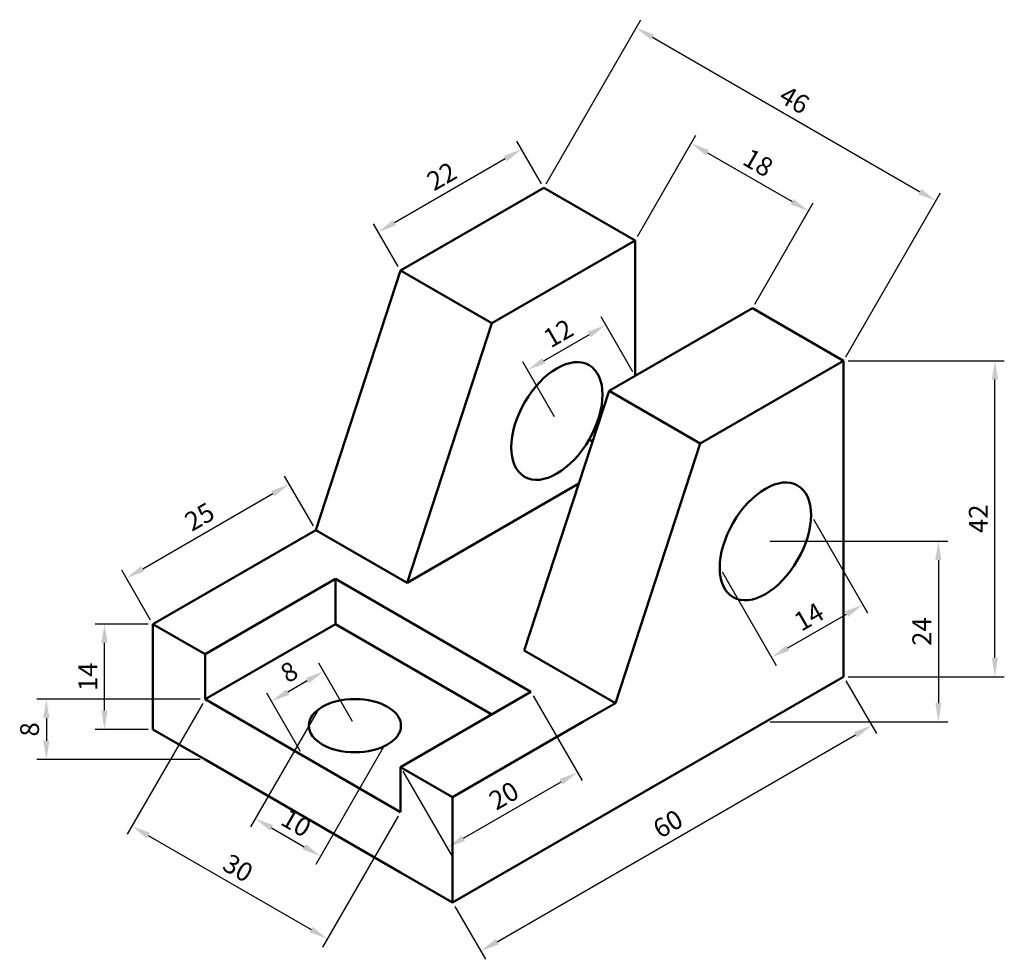
# Model space of a CAD drawing. Units: millimetres. Extents: x 1547 to 1678, y 118 to 243.
import ezdxf

# ---------------------------------------------------------------- set-up
doc = ezdxf.new("R2010")
doc.units = ezdxf.units.MM
doc.layers.add('M-DIMS', color=2, linetype='Continuous', lineweight=25)
doc.layers.add('M-OUTL', color=7, linetype='Continuous', lineweight=50)
doc.styles.get("Standard").update_dxf_attribs({"font": 'arial.ttf'})
doc.dimstyles.new('ISO-25', dxfattribs={"dimtxt": 2.5, "dimasz": 2.5, "dimexe": 1.25, "dimexo": 0.625, "dimtad": 1, "dimtxsty": 'Standard', "dimcen": 2.5, "dimadec": 0, "dimazin": 0, "dimtfac": 1, "dimtmove": 0, "dimatfit": 3, "dimfxl": 1, "dimarcsym": 0})

# ---------------------------------------------------------------- blocks, each defined once
blk = doc.blocks.new('*D1')
at = {"layer": 'Defpoints', "color": 0, "transparency": 16777216}
for p in [(1582.81, 181.09), (1586.33, 174.99), (1564.68, 162.49)]:
    blk.add_point(p, dxfattribs=at)
at = {"layer": 'M-DIMS', "color": 0, "lineweight": -2, "transparency": 16777216}
for p, q in [((1586.02, 175.53), (1582.18, 182.17)), ((1563.32, 169.84), (1580.64, 179.84)), ((1564.37, 163.03), (1560.53, 169.67))]:
    blk.add_line(p, q, dxfattribs=at)
at = {"layer": 'M-DIMS', "color": 0, "transparency": 16777216}
for points in [[(1580.44, 180.2), (1580.85, 179.48), (1582.81, 181.09)], [(1563.12, 170.2), (1563.53, 169.48), (1561.16, 168.59)]]:
    blk.add_solid(points, dxfattribs=at)
at = {"layer": 'M-DIMS', "color": 0, "transparency": 16777216, "insert": (1571.03, 176.48), "char_height": 2.5, "attachment_point": 5, "rotation": 30}
blk.add_mtext('25', dxfattribs=at)
blk = doc.blocks.new('*D2')
at = {"layer": 'Defpoints', "color": 0, "transparency": 16777216}
for p in [(1558.24, 162.49), (1564.68, 162.49), (1564.68, 148.49)]:
    blk.add_point(p, dxfattribs=at)
at = {"layer": 'M-DIMS', "color": 0, "lineweight": -2, "transparency": 16777216}
for p, q in [((1564.06, 162.49), (1556.99, 162.49)), ((1558.24, 150.99), (1558.24, 159.99)), ((1564.06, 148.49), (1556.99, 148.49))]:
    blk.add_line(p, q, dxfattribs=at)
at = {"layer": 'M-DIMS', "color": 0, "transparency": 16777216}
for points in [[(1557.82, 159.99), (1558.65, 159.99), (1558.24, 162.49)], [(1557.82, 150.99), (1558.65, 150.99), (1558.24, 148.49)]]:
    blk.add_solid(points, dxfattribs=at)
at = {"layer": 'M-DIMS', "color": 0, "transparency": 16777216, "insert": (1556.36, 155.49), "char_height": 2.5, "attachment_point": 5, "rotation": 90}
blk.add_mtext('14', dxfattribs=at)
blk = doc.blocks.new('*D3')
at = {"layer": 'Defpoints', "color": 0, "transparency": 16777216}
for p in [(1571.61, 152.49), (1550.52, 144.49), (1571.61, 144.49)]:
    blk.add_point(p, dxfattribs=at)
at = {"layer": 'M-DIMS', "color": 0, "lineweight": -2, "transparency": 16777216}
for p, q in [((1570.98, 152.49), (1549.27, 152.49)), ((1550.52, 149.99), (1550.52, 146.99)), ((1570.98, 144.49), (1549.27, 144.49))]:
    blk.add_line(p, q, dxfattribs=at)
at = {"layer": 'M-DIMS', "color": 0, "transparency": 16777216}
for points in [[(1550.1, 149.99), (1550.93, 149.99), (1550.52, 152.49)], [(1550.1, 146.99), (1550.93, 146.99), (1550.52, 144.49)]]:
    blk.add_solid(points, dxfattribs=at)
at = {"layer": 'M-DIMS', "color": 0, "transparency": 16777216, "insert": (1548.61, 148.49), "char_height": 2.5, "attachment_point": 5, "rotation": 90}
blk.add_mtext('8', dxfattribs=at)
blk = doc.blocks.new('*D4')
at = {"layer": 'Defpoints', "color": 0, "transparency": 16777216}
for p in [(1571.61, 152.49), (1597.59, 137.49), (1587.86, 120.64)]:
    blk.add_point(p, dxfattribs=at)
at = {"layer": 'M-DIMS', "color": 0, "lineweight": -2, "transparency": 16777216}
for p, q in [((1571.3, 151.94), (1561.26, 134.56)), ((1597.28, 136.94), (1587.24, 119.56)), ((1564.05, 134.39), (1585.7, 121.89))]:
    blk.add_line(p, q, dxfattribs=at)
at = {"layer": 'M-DIMS', "color": 0, "transparency": 16777216}
for points in [[(1564.26, 134.75), (1563.84, 134.03), (1561.88, 135.64)], [(1585.91, 122.25), (1585.49, 121.53), (1587.86, 120.64)]]:
    blk.add_solid(points, dxfattribs=at)
at = {"layer": 'M-DIMS', "color": 0, "transparency": 16777216, "insert": (1575.83, 129.79), "char_height": 2.5, "attachment_point": 5, "rotation": 330}
blk.add_mtext('30', dxfattribs=at)
blk = doc.blocks.new('*D5')
at = {"layer": 'Defpoints', "color": 0, "transparency": 16777216}
for p in [(1580.43, 152.2), (1591.53, 148.99), (1584.6, 144.99)]:
    blk.add_point(p, dxfattribs=at)
at = {"layer": 'M-DIMS', "color": 0, "lineweight": -2, "transparency": 16777216}
for p, q in [((1591.22, 149.53), (1586.74, 157.29)), ((1585.2, 154.95), (1582.6, 153.45)), ((1584.29, 145.53), (1579.81, 153.29))]:
    blk.add_line(p, q, dxfattribs=at)
at = {"layer": 'M-DIMS', "color": 0, "transparency": 16777216}
for points in [[(1584.99, 155.31), (1585.4, 154.59), (1587.36, 156.2)], [(1582.39, 153.81), (1582.81, 153.09), (1580.43, 152.2)]]:
    blk.add_solid(points, dxfattribs=at)
at = {"layer": 'M-DIMS', "color": 0, "transparency": 16777216, "insert": (1582.95, 155.85), "char_height": 2.5, "attachment_point": 5, "rotation": 30}
blk.add_mtext('8', dxfattribs=at)
blk = doc.blocks.new('*D6')
at = {"layer": 'Defpoints', "color": 0, "transparency": 16777216}
for p in [(1586.94, 151.63), (1595.6, 146.63), (1586.95, 131.64)]:
    blk.add_point(p, dxfattribs=at)
at = {"layer": 'M-DIMS', "color": 0, "lineweight": -2, "transparency": 16777216}
for p, q in [((1586.63, 151.09), (1577.66, 135.55)), ((1595.29, 146.09), (1586.32, 130.55)), ((1580.45, 135.39), (1584.78, 132.89))]:
    blk.add_line(p, q, dxfattribs=at)
at = {"layer": 'M-DIMS', "color": 0, "transparency": 16777216}
for points in [[(1580.66, 135.75), (1580.24, 135.03), (1578.29, 136.64)], [(1584.99, 133.25), (1584.57, 132.53), (1586.95, 131.64)]]:
    blk.add_solid(points, dxfattribs=at)
at = {"layer": 'M-DIMS', "color": 0, "transparency": 16777216, "insert": (1583.57, 135.78), "char_height": 2.5, "attachment_point": 5, "rotation": 330}
blk.add_mtext('10', dxfattribs=at)
blk = doc.blocks.new('*D7')
at = {"layer": 'Defpoints', "color": 0, "transparency": 16777216}
for p in [(1656.48, 155.49), (1660.22, 149.01), (1604.52, 125.49)]:
    blk.add_point(p, dxfattribs=at)
at = {"layer": 'M-DIMS', "color": 0, "lineweight": -2, "transparency": 16777216}
for p, q in [((1656.79, 154.94), (1660.85, 147.93)), ((1610.42, 120.26), (1658.06, 147.76)), ((1604.83, 124.94), (1608.88, 117.93))]:
    blk.add_line(p, q, dxfattribs=at)
at = {"layer": 'M-DIMS', "color": 0, "transparency": 16777216}
for points in [[(1657.85, 148.12), (1658.26, 147.4), (1660.22, 149.01)], [(1610.22, 120.62), (1610.63, 119.9), (1608.26, 119.01)]]:
    blk.add_solid(points, dxfattribs=at)
at = {"layer": 'M-DIMS', "color": 0, "transparency": 16777216, "insert": (1633.29, 135.66), "char_height": 2.5, "attachment_point": 5, "rotation": 30}
blk.add_mtext('60', dxfattribs=at)
blk = doc.blocks.new('*D8')
at = {"layer": 'Defpoints', "color": 0, "transparency": 16777216}
for p in [(1656.48, 197.49), (1676.59, 197.49), (1656.48, 155.49)]:
    blk.add_point(p, dxfattribs=at)
at = {"layer": 'M-DIMS', "color": 0, "lineweight": -2, "transparency": 16777216}
for p, q in [((1657.11, 197.49), (1677.84, 197.49)), ((1676.59, 157.99), (1676.59, 194.99)), ((1657.11, 155.49), (1677.84, 155.49))]:
    blk.add_line(p, q, dxfattribs=at)
at = {"layer": 'M-DIMS', "color": 0, "transparency": 16777216}
for points in [[(1676.18, 194.99), (1677.01, 194.99), (1676.59, 197.49)], [(1676.18, 157.99), (1677.01, 157.99), (1676.59, 155.49)]]:
    blk.add_solid(points, dxfattribs=at)
at = {"layer": 'M-DIMS', "color": 0, "transparency": 16777216, "insert": (1674.71, 176.49), "char_height": 2.5, "attachment_point": 5, "rotation": 90}
blk.add_mtext('42', dxfattribs=at)
blk = doc.blocks.new('*D9')
at = {"layer": 'Defpoints', "color": 0, "transparency": 16777216}
for p in [(1652.15, 176.99), (1640.03, 169.99), (1659.03, 165.06)]:
    blk.add_point(p, dxfattribs=at)
at = {"layer": 'M-DIMS', "color": 0, "lineweight": -2, "transparency": 16777216}
for p, q in [((1652.46, 176.44), (1659.66, 163.98)), ((1640.34, 169.44), (1647.53, 156.98)), ((1649.07, 159.31), (1656.87, 163.81))]:
    blk.add_line(p, q, dxfattribs=at)
at = {"layer": 'M-DIMS', "color": 0, "transparency": 16777216}
for points in [[(1656.66, 164.18), (1657.08, 163.45), (1659.03, 165.06)], [(1648.87, 159.68), (1649.28, 158.95), (1646.91, 158.06)]]:
    blk.add_solid(points, dxfattribs=at)
at = {"layer": 'M-DIMS', "color": 0, "transparency": 16777216, "insert": (1652.03, 163.19), "char_height": 2.5, "attachment_point": 5, "rotation": 30}
blk.add_mtext('14', dxfattribs=at)
blk = doc.blocks.new('*D10')
at = {"layer": 'Defpoints', "color": 0, "transparency": 16777216}
for p in [(1613.68, 225.61), (1616.64, 220.49), (1597.59, 209.49)]:
    blk.add_point(p, dxfattribs=at)
at = {"layer": 'M-DIMS', "color": 0, "lineweight": -2, "transparency": 16777216}
for p, q in [((1616.33, 221.03), (1613.06, 226.7)), ((1596.8, 215.86), (1611.52, 224.36)), ((1597.28, 210.03), (1594.01, 215.7))]:
    blk.add_line(p, q, dxfattribs=at)
at = {"layer": 'M-DIMS', "color": 0, "transparency": 16777216}
for points in [[(1611.31, 224.72), (1611.73, 224), (1613.68, 225.61)], [(1596.59, 216.22), (1597, 215.5), (1594.63, 214.61)]]:
    blk.add_solid(points, dxfattribs=at)
at = {"layer": 'M-DIMS', "color": 0, "transparency": 16777216, "insert": (1603.22, 221.74), "char_height": 2.5, "attachment_point": 5, "rotation": 30}
blk.add_mtext('22', dxfattribs=at)
blk = doc.blocks.new('*D11')
at = {"layer": 'Defpoints', "color": 0, "transparency": 16777216}
for p in [(1624.86, 202.25), (1628.77, 195.49), (1618.38, 189.49)]:
    blk.add_point(p, dxfattribs=at)
at = {"layer": 'M-DIMS', "color": 0, "lineweight": -2, "transparency": 16777216}
for p, q in [((1628.46, 196.03), (1624.24, 203.33)), ((1616.64, 197.5), (1622.7, 201)), ((1618.06, 190.03), (1613.85, 197.33))]:
    blk.add_line(p, q, dxfattribs=at)
at = {"layer": 'M-DIMS', "color": 0, "transparency": 16777216}
for points in [[(1622.49, 201.36), (1622.91, 200.64), (1624.86, 202.25)], [(1616.43, 197.86), (1616.85, 197.14), (1614.47, 196.25)]]:
    blk.add_solid(points, dxfattribs=at)
at = {"layer": 'M-DIMS', "color": 0, "transparency": 16777216, "insert": (1618.73, 200.87), "char_height": 2.5, "attachment_point": 5, "rotation": 30}
blk.add_mtext('12', dxfattribs=at)
blk = doc.blocks.new('*D12')
at = {"layer": 'Defpoints', "color": 0, "transparency": 16777216}
for p in [(1651.81, 217.4), (1628.77, 213.49), (1644.36, 204.49)]:
    blk.add_point(p, dxfattribs=at)
at = {"layer": 'M-DIMS', "color": 0, "lineweight": -2, "transparency": 16777216}
for p, q in [((1629.08, 214.03), (1636.85, 227.48)), ((1638.39, 225.15), (1649.65, 218.65)), ((1644.67, 205.03), (1652.44, 218.48))]:
    blk.add_line(p, q, dxfattribs=at)
at = {"layer": 'M-DIMS', "color": 0, "transparency": 16777216}
for points in [[(1638.6, 225.51), (1638.18, 224.79), (1636.22, 226.4)], [(1649.86, 219.01), (1649.44, 218.29), (1651.81, 217.4)]]:
    blk.add_solid(points, dxfattribs=at)
at = {"layer": 'M-DIMS', "color": 0, "transparency": 16777216, "insert": (1644.97, 223.55), "char_height": 2.5, "attachment_point": 5, "rotation": 330}
blk.add_mtext('18', dxfattribs=at)
blk = doc.blocks.new('*D13')
at = {"layer": 'Defpoints', "color": 0, "transparency": 16777216}
for p in [(1616.64, 220.49), (1668.76, 218.75), (1656.48, 197.49)]:
    blk.add_point(p, dxfattribs=at)
at = {"layer": 'M-DIMS', "color": 0, "lineweight": -2, "transparency": 16777216}
for p, q in [((1616.96, 221.03), (1629.55, 242.83)), ((1631.09, 240.5), (1666.59, 220)), ((1656.79, 198.03), (1669.38, 219.83))]:
    blk.add_line(p, q, dxfattribs=at)
at = {"layer": 'M-DIMS', "color": 0, "transparency": 16777216}
for points in [[(1631.29, 240.86), (1630.88, 240.14), (1628.92, 241.75)], [(1666.8, 220.36), (1666.38, 219.64), (1668.76, 218.75)]]:
    blk.add_solid(points, dxfattribs=at)
at = {"layer": 'M-DIMS', "color": 0, "transparency": 16777216, "insert": (1649.79, 231.9), "char_height": 2.5, "attachment_point": 5, "rotation": 330}
blk.add_mtext('46', dxfattribs=at)
blk = doc.blocks.new('*D14')
at = {"layer": 'Defpoints', "color": 0, "transparency": 16777216}
for p in [(1646.09, 173.49), (1646.09, 149.49), (1669.08, 149.49)]:
    blk.add_point(p, dxfattribs=at)
at = {"layer": 'M-DIMS', "color": 0, "lineweight": -2, "transparency": 16777216}
for p, q in [((1646.71, 173.49), (1670.33, 173.49)), ((1669.08, 170.99), (1669.08, 151.99)), ((1646.71, 149.49), (1670.33, 149.49))]:
    blk.add_line(p, q, dxfattribs=at)
at = {"layer": 'M-DIMS', "color": 0, "transparency": 16777216}
for points in [[(1668.66, 170.99), (1669.5, 170.99), (1669.08, 173.49)], [(1668.66, 151.99), (1669.5, 151.99), (1669.08, 149.49)]]:
    blk.add_solid(points, dxfattribs=at)
at = {"layer": 'M-DIMS', "color": 0, "transparency": 16777216, "insert": (1667.2, 161.49), "char_height": 2.5, "attachment_point": 5, "rotation": 90}
blk.add_mtext('24', dxfattribs=at)
blk = doc.blocks.new('*D15')
at = {"layer": 'Defpoints', "color": 0, "transparency": 16777216}
for p in [(1614.91, 153.49), (1597.59, 143.49), (1621.1, 142.77)]:
    blk.add_point(p, dxfattribs=at)
at = {"layer": 'M-DIMS', "color": 0, "lineweight": -2, "transparency": 16777216}
for p, q in [((1615.22, 152.94), (1621.73, 141.68)), ((1597.9, 142.94), (1604.41, 131.68)), ((1605.95, 134.02), (1618.94, 141.52))]:
    blk.add_line(p, q, dxfattribs=at)
at = {"layer": 'M-DIMS', "color": 0, "transparency": 16777216}
for points in [[(1618.73, 141.88), (1619.14, 141.15), (1621.1, 142.77)], [(1605.74, 134.38), (1606.15, 133.65), (1603.78, 132.77)]]:
    blk.add_solid(points, dxfattribs=at)
at = {"layer": 'M-DIMS', "color": 0, "transparency": 16777216, "insert": (1611.49, 139.41), "char_height": 2.5, "attachment_point": 5, "rotation": 30}
blk.add_mtext('20', dxfattribs=at)

msp = doc.modelspace()

# ---------------------------------------------------------------- linework, layer by layer
at = {"layer": 'M-OUTL'}
for p, q in [((1597.591, 209.486), (1616.643, 220.486)), ((1616.643, 220.486), (1628.768, 213.486)), ((1628.768, 213.486), (1609.715, 202.486)), ((1628.768, 213.486), (1628.768, 195.486)), ((1586.332, 174.986), (1597.591, 209.486)), ((1609.715, 202.486), (1597.591, 209.486)), ((1644.356, 204.486), (1625.304, 193.486)), ((1656.48, 197.486), (1644.356, 204.486)), ((1598.457, 167.986), (1609.715, 202.486)), ((1637.428, 186.486), (1656.48, 197.486)), ((1656.48, 155.486), (1656.48, 197.486)), ((1625.304, 193.486), (1614.045, 158.986)), ((1625.304, 193.486), (1637.428, 186.486)), ((1623.107, 186.754), (1622.662, 187.011)), ((1626.17, 151.986), (1637.428, 186.486)), ((1598.457, 167.986), (1621.283, 181.165)), ((1621.283, 181.165), (1621.283, 181.165)), ((1564.682, 162.486), (1586.332, 174.986)), ((1586.332, 174.986), (1598.457, 167.986)), ((1588.93, 168.486), (1571.61, 158.486)), ((1614.911, 153.486), (1588.93, 168.486)), ((1588.93, 168.486), (1588.93, 162.486)), ((1564.682, 148.486), (1564.682, 162.486)), ((1564.682, 162.486), (1571.61, 158.486)), ((1571.61, 152.486), (1588.93, 162.486)), ((1588.93, 162.486), (1609.715, 150.486)), ((1571.61, 152.486), (1571.61, 158.486)), ((1626.17, 151.986), (1614.045, 158.986)), ((1604.519, 125.486), (1656.48, 155.486)), ((1597.591, 143.486), (1614.911, 153.486)), ((1597.591, 137.486), (1571.61, 152.486)), ((1621.839, 149.486), (1626.17, 151.986)), ((1604.519, 139.486), (1621.839, 149.486)), ((1571.61, 144.486), (1564.682, 148.486)), ((1597.591, 129.486), (1571.61, 144.486)), ((1597.591, 143.486), (1604.519, 139.486)), ((1597.591, 137.486), (1597.591, 143.486)), ((1604.519, 125.486), (1604.519, 139.486)), ((1604.519, 125.486), (1597.591, 129.486))]:
    msp.add_line(p, q, dxfattribs=at)
for centre, major_axis in [((1618.375, 189.486), (-4.287, -7.425)), ((1646.088, 173.486), (-4.287, -7.425)), ((1591.529, 148.986), (-6.124, 0))]:
    msp.add_ellipse(centre, major_axis=major_axis, ratio=0.5773503, dxfattribs=at)

# ---------------------------------------------------------------- dimensions: what is measured, and where the dimension line sits
at = {"layer": 'M-DIMS'}
for p1, p2, distance, picture, middle in [((1616.643, 220.486), (1656.48, 197.486), 24.554, '*D13', (1649.79, 231.897)), ((1597.591, 209.486), (1616.643, 220.486), 5.921, '*D10', (1603.217, 221.742)), ((1628.768, 213.486), (1644.356, 204.486), 14.914, '*D12', (1644.969, 223.548)), ((1618.375, 189.486), (1628.768, 195.486), 7.806, '*D11', (1618.728, 200.875)), ((1564.682, 162.486), (1586.332, 174.986), 7.046, '*D1', (1571.034, 176.484)), ((1640.026, 169.986), (1652.15, 176.986), -13.765, '*D9', (1652.031, 163.193)), ((1591.529, 148.986), (1584.6, 144.986), -8.334, '*D5', (1582.947, 155.85)), ((1604.519, 125.486), (1656.48, 155.486), -7.48, '*D7', (1633.289, 135.655)), ((1597.591, 143.486), (1614.911, 153.486), -12.379, '*D15', (1611.49, 139.412)), ((1571.61, 152.486), (1597.591, 137.486), -19.452, '*D4', (1575.825, 129.787)), ((1586.944, 151.633), (1595.604, 146.633), -17.316, '*D6', (1583.567, 135.783))]:
    dim = msp.add_aligned_dim(p1=p1, p2=p2, distance=distance, dimstyle='ISO-25', override={"dimclrd": 0, "dimclre": 0, "dimclrt": 0}, dxfattribs=at)
    dim.commit()
    dim.dimension.update_dxf_attribs({"geometry": picture, "text_midpoint": middle})
for base, p1, p2, picture, middle in [((1676.593, 197.486), (1656.48, 155.486), (1656.48, 197.486), '*D8', (1674.713, 176.486)), ((1669.079, 149.486), (1646.088, 173.486), (1646.088, 149.486), '*D14', (1667.199, 161.486)), ((1558.235, 162.486), (1564.682, 148.486), (1564.682, 162.486), '*D2', (1556.355, 155.486)), ((1550.516, 144.486), (1571.61, 152.486), (1571.61, 144.486), '*D3', (1548.615, 148.486))]:
    dim = msp.add_linear_dim(base=base, p1=p1, p2=p2, angle=90, dimstyle='ISO-25', override={"dimclrd": 0, "dimclre": 0, "dimclrt": 0}, dxfattribs=at)
    dim.commit()
    dim.dimension.update_dxf_attribs({"geometry": picture, "text_midpoint": middle})

doc.saveas('drawing.dxf')
